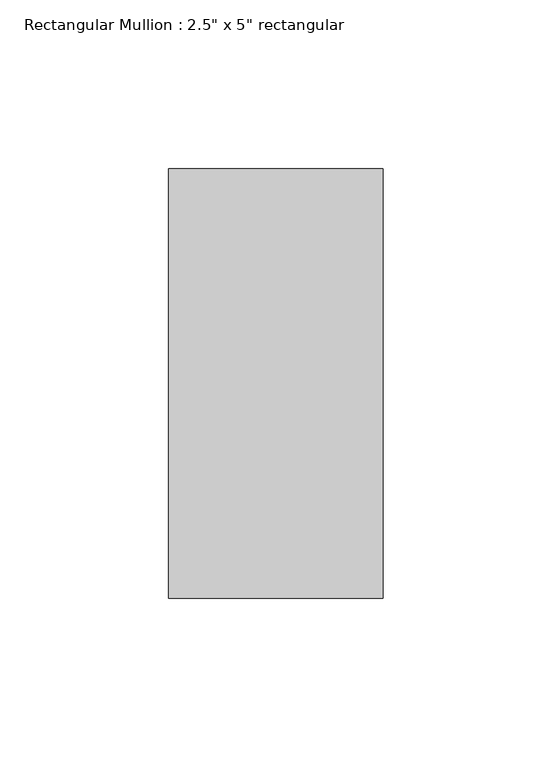
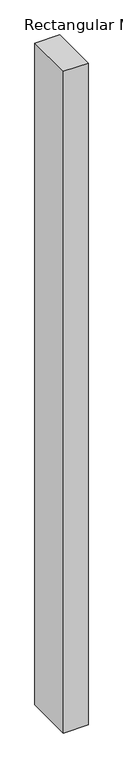
"""IFC4 building model written with IfcOpenShell, lengths in millimetres: member geometry."""

from ifc_helpers import new_model, si_unit, frame, origin, place, context, project, spatial, polyline, outline, extrude, source, transform, mapped, element, save


def member_5a9e6520(model_context):
    return source(origin(), model_context, "Body", "SweptSolid", [
        extrude(outline(polyline([(0.0, 63.5), (0.0, -63.5), (-63.5, -63.5), (-63.5, 63.5), (0.0, 63.5)])), frame((0.0, 0.0, -1801.1599467), z_axis=(0.0, 0.0, 1.0), x_axis=(1.0, 0.0, 0.0)), (0.0, 0.0, 1.0), 1801.1599467),
    ])


if __name__ == "__main__":
    model = new_model("IFC4")
    model_context = context("Model", 3, world=origin())
    ifc_project = project(units=[si_unit("LENGTHUNIT", "METRE", prefix="MILLI")], contexts=[model_context])
    site = spatial("IfcSite", under=ifc_project)
    building = spatial("IfcBuilding", under=site)
    placement = place(None, origin())
    member_shape = member_5a9e6520(model_context)
    element("IfcMember", 1, ObjectType="Rectangular Mullion : 2.5\" x 5\" rectangular", at=placement, inside=building, context=model_context, shape_type="MappedRepresentation", body=[
        mapped(member_shape, transform((0.0, 0.0, 0.0), x_axis=(1.0, 0.0, 0.0), y_axis=(0.0, 1.0, 0.0), z_axis=(0.0, 0.0, 1.0))),
    ])
    save(model, "model.ifc")

# Revit data of these elements
# Type "Rectangular Mullion : 2.5\" x 5\" rectangular"
#   built-in parameter 1007304 = 0.416667 (stored number, unit not read)
#   built-in parameter 1007301 = 0.104167 (stored number, unit not read)
#   built-in parameter 1007300 = 0.104167 (stored number, unit not read)
# Element 1 (IfcMember, "Rectangular Mullion : 2.5\" x 5\" rectangular")
#   Materials on its faces: "Aluminum"
# Materials
#   "Aluminum": class "Metal", colour RGB 247 247 247, transparency 0, Description = "Aluminum 6061", Cost = 0
